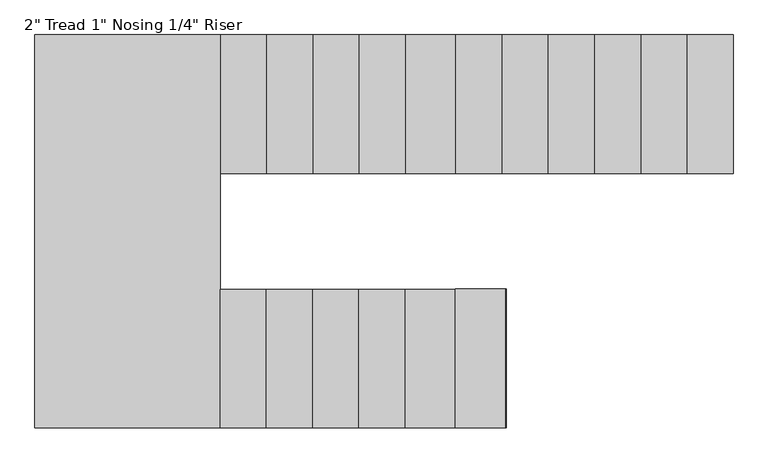
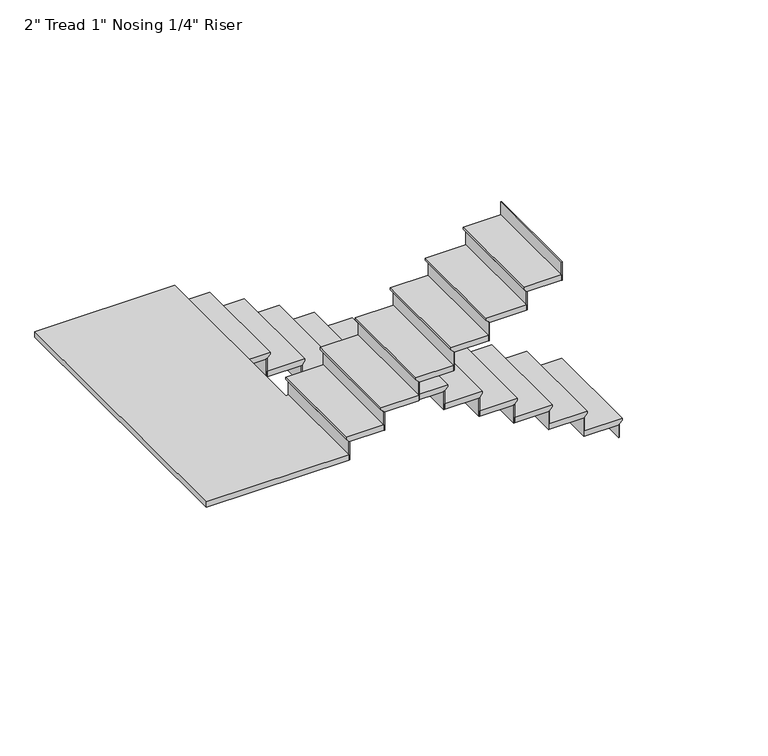
"""IFC4 building model written with IfcOpenShell, lengths in millimetres: stair flight geometry."""

from ifc_helpers import new_model, si_unit, origin, place, context, project, spatial, faceted_brep, source, transform, mapped, element, save


def stair_flight_6b31ae14(model_context):
    return source(origin(), model_context, "Body", "Brep", [
        faceted_brep([(10969.6546318, 8847.834892, 149.3921053), (10969.6546318, 8847.834892, 168.4421053), (10969.6546318, 7933.434892, 168.4421053), (10969.6546318, 7933.434892, 149.3921053), (10944.2546318, 8847.834892, 123.9921053), (10944.2546318, 7933.434892, 123.9921053), (10639.4546318, 8847.834892, 168.4421053), (10639.4546318, 7933.434892, 168.4421053), (10944.2546318, 7933.434892, 117.6421053), (10639.4546318, 7933.434892, 117.6421053), (10639.4546318, 8847.834892, 117.6421053), (10944.2546318, 8847.834892, 117.6421053)], [[[0, 1, 2, 3]], [[4, 0, 3, 5]], [[2, 1, 6, 7]], [[8, 9, 10, 11]], [[2, 7, 9, 8, 5, 3]], [[8, 11, 4, 5]], [[6, 1, 0, 4, 11, 10]], [[7, 6, 10, 9]]]),
        faceted_brep([(10944.2546318, 8847.834892, 117.6421053), (10944.2546318, 8847.834892, 0.0), (10937.9046318, 8847.834892, 0.0), (10937.9046318, 8847.834892, 117.6421053), (10944.2546318, 7933.434892, 117.6421053), (10937.9046318, 7933.434892, 117.6421053), (10937.9046318, 7933.434892, 0.0), (10944.2546318, 7933.434892, 0.0)], [[[0, 1, 2, 3]], [[4, 5, 6, 7]], [[1, 0, 4, 7]], [[2, 1, 7, 6]], [[3, 2, 6, 5]], [[0, 3, 5, 4]]]),
        faceted_brep([(10639.4546318, 8847.834892, 286.0842105), (10639.4546318, 8847.834892, 117.6421053), (10633.1046318, 8847.834892, 117.6421053), (10633.1046318, 8847.834892, 286.0842105), (10639.4546318, 7933.434892, 286.0842105), (10633.1046318, 7933.434892, 286.0842105), (10633.1046318, 7933.434892, 117.6421053), (10639.4546318, 7933.434892, 117.6421053)], [[[0, 1, 2, 3]], [[4, 5, 6, 7]], [[1, 0, 4, 7]], [[2, 1, 7, 6]], [[3, 2, 6, 5]], [[0, 3, 5, 4]]]),
        faceted_brep([(10664.8546318, 7933.434892, 336.8842105), (10664.8546318, 8847.834892, 336.8842105), (10334.6546318, 8847.834892, 336.8842105), (10334.6546318, 7933.434892, 336.8842105), (10639.4546318, 7933.434892, 286.0842105), (10334.6546318, 7933.434892, 286.0842105), (10334.6546318, 8847.834892, 286.0842105), (10639.4546318, 8847.834892, 286.0842105), (10639.4546318, 7933.434892, 292.4342105), (10664.8546318, 7933.434892, 317.8342105), (10639.4546318, 8847.834892, 292.4342105), (10664.8546318, 8847.834892, 317.8342105)], [[[0, 1, 2, 3]], [[4, 5, 6, 7]], [[0, 3, 5, 4, 8, 9]], [[4, 7, 10, 8]], [[2, 1, 11, 10, 7, 6]], [[3, 2, 6, 5]], [[11, 1, 0, 9]], [[10, 11, 9, 8]]]),
        faceted_brep([(10334.6546318, 8847.834892, 454.5263158), (10334.6546318, 8847.834892, 286.0842105), (10328.3046318, 8847.834892, 286.0842105), (10328.3046318, 8847.834892, 454.5263158), (10334.6546318, 7933.434892, 454.5263158), (10328.3046318, 7933.434892, 454.5263158), (10328.3046318, 7933.434892, 286.0842105), (10334.6546318, 7933.434892, 286.0842105)], [[[0, 1, 2, 3]], [[4, 5, 6, 7]], [[1, 0, 4, 7]], [[2, 1, 7, 6]], [[3, 2, 6, 5]], [[0, 3, 5, 4]]]),
        faceted_brep([(10360.0546318, 7933.434892, 505.3263158), (10360.0546318, 8847.834892, 505.3263158), (10029.8546318, 8847.834892, 505.3263158), (10029.8546318, 7933.434892, 505.3263158), (10334.6546318, 7933.434892, 454.5263158), (10029.8546318, 7933.434892, 454.5263158), (10029.8546318, 8847.834892, 454.5263158), (10334.6546318, 8847.834892, 454.5263158), (10334.6546318, 7933.434892, 460.8763158), (10360.0546318, 7933.434892, 486.2763158), (10334.6546318, 8847.834892, 460.8763158), (10360.0546318, 8847.834892, 486.2763158)], [[[0, 1, 2, 3]], [[4, 5, 6, 7]], [[0, 3, 5, 4, 8, 9]], [[4, 7, 10, 8]], [[2, 1, 11, 10, 7, 6]], [[3, 2, 6, 5]], [[11, 1, 0, 9]], [[10, 11, 9, 8]]]),
        faceted_brep([(10029.8546318, 8847.834892, 622.9684211), (10029.8546318, 8847.834892, 454.5263158), (10023.5046318, 8847.834892, 454.5263158), (10023.5046318, 8847.834892, 622.9684211), (10029.8546318, 7933.434892, 622.9684211), (10023.5046318, 7933.434892, 622.9684211), (10023.5046318, 7933.434892, 454.5263158), (10029.8546318, 7933.434892, 454.5263158)], [[[0, 1, 2, 3]], [[4, 5, 6, 7]], [[1, 0, 4, 7]], [[2, 1, 7, 6]], [[3, 2, 6, 5]], [[0, 3, 5, 4]]]),
        faceted_brep([(10055.2546318, 7933.434892, 673.7684211), (10055.2546318, 8847.834892, 673.7684211), (9725.0546318, 8847.834892, 673.7684211), (9725.0546318, 7933.434892, 673.7684211), (10029.8546318, 7933.434892, 622.9684211), (9725.0546318, 7933.434892, 622.9684211), (9725.0546318, 8847.834892, 622.9684211), (10029.8546318, 8847.834892, 622.9684211), (10029.8546318, 7933.434892, 629.3184211), (10055.2546318, 7933.434892, 654.7184211), (10029.8546318, 8847.834892, 629.3184211), (10055.2546318, 8847.834892, 654.7184211)], [[[0, 1, 2, 3]], [[4, 5, 6, 7]], [[0, 3, 5, 4, 8, 9]], [[4, 7, 10, 8]], [[2, 1, 11, 10, 7, 6]], [[3, 2, 6, 5]], [[11, 1, 0, 9]], [[10, 11, 9, 8]]]),
        faceted_brep([(9725.0546318, 8847.834892, 791.4105263), (9725.0546318, 8847.834892, 622.9684211), (9718.7046318, 8847.834892, 622.9684211), (9718.7046318, 8847.834892, 791.4105263), (9725.0546318, 7933.434892, 791.4105263), (9718.7046318, 7933.434892, 791.4105263), (9718.7046318, 7933.434892, 622.9684211), (9725.0546318, 7933.434892, 622.9684211)], [[[0, 1, 2, 3]], [[4, 5, 6, 7]], [[1, 0, 4, 7]], [[2, 1, 7, 6]], [[3, 2, 6, 5]], [[0, 3, 5, 4]]]),
        faceted_brep([(9750.4546318, 7933.434892, 842.2105263), (9750.4546318, 8847.834892, 842.2105263), (9420.2546318, 8847.834892, 842.2105263), (9420.2546318, 7933.434892, 842.2105263), (9725.0546318, 7933.434892, 791.4105263), (9420.2546318, 7933.434892, 791.4105263), (9420.2546318, 8847.834892, 791.4105263), (9725.0546318, 8847.834892, 791.4105263), (9725.0546318, 7933.434892, 797.7605263), (9750.4546318, 7933.434892, 823.1605263), (9725.0546318, 8847.834892, 797.7605263), (9750.4546318, 8847.834892, 823.1605263)], [[[0, 1, 2, 3]], [[4, 5, 6, 7]], [[0, 3, 5, 4, 8, 9]], [[4, 7, 10, 8]], [[2, 1, 11, 10, 7, 6]], [[3, 2, 6, 5]], [[11, 1, 0, 9]], [[10, 11, 9, 8]]]),
        faceted_brep([(9420.2546318, 8847.834892, 959.8526316), (9420.2546318, 8847.834892, 791.4105263), (9413.9046318, 8847.834892, 791.4105263), (9413.9046318, 8847.834892, 959.8526316), (9420.2546318, 7933.434892, 959.8526316), (9413.9046318, 7933.434892, 959.8526316), (9413.9046318, 7933.434892, 791.4105263), (9420.2546318, 7933.434892, 791.4105263)], [[[0, 1, 2, 3]], [[4, 5, 6, 7]], [[1, 0, 4, 7]], [[2, 1, 7, 6]], [[3, 2, 6, 5]], [[0, 3, 5, 4]]]),
        faceted_brep([(9445.6546318, 7933.434892, 1010.6526316), (9445.6546318, 8847.834892, 1010.6526316), (9115.4546318, 8847.834892, 1010.6526316), (9115.4546318, 7933.434892, 1010.6526316), (9420.2546318, 7933.434892, 959.8526316), (9115.4546318, 7933.434892, 959.8526316), (9115.4546318, 8847.834892, 959.8526316), (9420.2546318, 8847.834892, 959.8526316), (9420.2546318, 7933.434892, 966.2026316), (9445.6546318, 7933.434892, 991.6026316), (9420.2546318, 8847.834892, 966.2026316), (9445.6546318, 8847.834892, 991.6026316)], [[[0, 1, 2, 3]], [[4, 5, 6, 7]], [[0, 3, 5, 4, 8, 9]], [[4, 7, 10, 8]], [[2, 1, 11, 10, 7, 6]], [[3, 2, 6, 5]], [[11, 1, 0, 9]], [[10, 11, 9, 8]]]),
        faceted_brep([(9115.4546318, 8847.834892, 1128.2947368), (9115.4546318, 8847.834892, 959.8526316), (9109.1046318, 8847.834892, 959.8526316), (9109.1046318, 8847.834892, 1128.2947368), (9115.4546318, 7933.434892, 1128.2947368), (9109.1046318, 7933.434892, 1128.2947368), (9109.1046318, 7933.434892, 959.8526316), (9115.4546318, 7933.434892, 959.8526316)], [[[0, 1, 2, 3]], [[4, 5, 6, 7]], [[1, 0, 4, 7]], [[2, 1, 7, 6]], [[3, 2, 6, 5]], [[0, 3, 5, 4]]]),
        faceted_brep([(9140.8546318, 7933.434892, 1179.0947368), (9140.8546318, 8847.834892, 1179.0947368), (8785.2546318, 8847.834892, 1179.0947368), (8785.2546318, 7933.434892, 1179.0947368), (9115.4546318, 7933.434892, 1128.2947368), (8785.2546318, 7933.434892, 1128.2947368), (8785.2546318, 8847.834892, 1128.2947368), (9115.4546318, 8847.834892, 1128.2947368), (9115.4546318, 7933.434892, 1134.6447368), (9140.8546318, 7933.434892, 1160.0447368), (9115.4546318, 8847.834892, 1134.6447368), (9140.8546318, 8847.834892, 1160.0447368)], [[[0, 1, 2, 3]], [[4, 5, 6, 7]], [[0, 3, 5, 4, 8, 9]], [[4, 7, 10, 8]], [[2, 1, 11, 10, 7, 6]], [[3, 2, 6, 5]], [[11, 1, 0, 9]], [[10, 11, 9, 8]]]),
        faceted_brep([(8785.2546318, 8847.834892, 1296.7368421), (8785.2546318, 8847.834892, 1128.2947368), (8778.9046318, 8847.834892, 1128.2947368), (8778.9046318, 8847.834892, 1296.7368421), (8785.2546318, 7933.434892, 1296.7368421), (8778.9046318, 7933.434892, 1296.7368421), (8778.9046318, 7933.434892, 1128.2947368), (8785.2546318, 7933.434892, 1128.2947368)], [[[0, 1, 2, 3]], [[4, 5, 6, 7]], [[1, 0, 4, 7]], [[2, 1, 7, 6]], [[3, 2, 6, 5]], [[0, 3, 5, 4]]]),
        faceted_brep([(8810.6546318, 7933.434892, 1347.5368421), (8810.6546318, 8847.834892, 1347.5368421), (8480.4546318, 8847.834892, 1347.5368421), (8480.4546318, 7933.434892, 1347.5368421), (8785.2546318, 7933.434892, 1296.7368421), (8480.4546318, 7933.434892, 1296.7368421), (8480.4546318, 8847.834892, 1296.7368421), (8785.2546318, 8847.834892, 1296.7368421), (8785.2546318, 7933.434892, 1303.0868421), (8810.6546318, 7933.434892, 1328.4868421), (8785.2546318, 8847.834892, 1303.0868421), (8810.6546318, 8847.834892, 1328.4868421)], [[[0, 1, 2, 3]], [[4, 5, 6, 7]], [[0, 3, 5, 4, 8, 9]], [[4, 7, 10, 8]], [[2, 1, 11, 10, 7, 6]], [[3, 2, 6, 5]], [[11, 1, 0, 9]], [[10, 11, 9, 8]]]),
        faceted_brep([(8480.4546318, 8847.834892, 1465.1789474), (8480.4546318, 8847.834892, 1296.7368421), (8474.1046318, 8847.834892, 1296.7368421), (8474.1046318, 8847.834892, 1465.1789474), (8480.4546318, 7933.434892, 1465.1789474), (8474.1046318, 7933.434892, 1465.1789474), (8474.1046318, 7933.434892, 1296.7368421), (8480.4546318, 7933.434892, 1296.7368421)], [[[0, 1, 2, 3]], [[4, 5, 6, 7]], [[1, 0, 4, 7]], [[2, 1, 7, 6]], [[3, 2, 6, 5]], [[0, 3, 5, 4]]]),
        faceted_brep([(8505.8546318, 7933.434892, 1515.9789474), (8505.8546318, 8847.834892, 1515.9789474), (8175.6546318, 8847.834892, 1515.9789474), (8175.6546318, 7933.434892, 1515.9789474), (8480.4546318, 7933.434892, 1465.1789474), (8175.6546318, 7933.434892, 1465.1789474), (8175.6546318, 8847.834892, 1465.1789474), (8480.4546318, 8847.834892, 1465.1789474), (8480.4546318, 7933.434892, 1471.5289474), (8505.8546318, 7933.434892, 1496.9289474), (8480.4546318, 8847.834892, 1471.5289474), (8505.8546318, 8847.834892, 1496.9289474)], [[[0, 1, 2, 3]], [[4, 5, 6, 7]], [[0, 3, 5, 4, 8, 9]], [[4, 7, 10, 8]], [[2, 1, 11, 10, 7, 6]], [[3, 2, 6, 5]], [[11, 1, 0, 9]], [[10, 11, 9, 8]]]),
        faceted_brep([(8175.6546318, 8847.834892, 1633.6210526), (8175.6546318, 8847.834892, 1465.1789474), (8169.3046318, 8847.834892, 1465.1789474), (8169.3046318, 8847.834892, 1633.6210526), (8175.6546318, 7933.434892, 1633.6210526), (8169.3046318, 7933.434892, 1633.6210526), (8169.3046318, 7933.434892, 1465.1789474), (8175.6546318, 7933.434892, 1465.1789474)], [[[0, 1, 2, 3]], [[4, 5, 6, 7]], [[1, 0, 4, 7]], [[2, 1, 7, 6]], [[3, 2, 6, 5]], [[0, 3, 5, 4]]]),
        faceted_brep([(8201.0546318, 7933.434892, 1684.4210526), (8201.0546318, 8847.834892, 1684.4210526), (7870.8546318, 8847.834892, 1684.4210526), (7870.8546318, 7933.434892, 1684.4210526), (8175.6546318, 7933.434892, 1633.6210526), (7870.8546318, 7933.434892, 1633.6210526), (7870.8546318, 8847.834892, 1633.6210526), (8175.6546318, 8847.834892, 1633.6210526), (8175.6546318, 7933.434892, 1639.9710526), (8201.0546318, 7933.434892, 1665.3710526), (8175.6546318, 8847.834892, 1639.9710526), (8201.0546318, 8847.834892, 1665.3710526)], [[[0, 1, 2, 3]], [[4, 5, 6, 7]], [[0, 3, 5, 4, 8, 9]], [[4, 7, 10, 8]], [[2, 1, 11, 10, 7, 6]], [[3, 2, 6, 5]], [[11, 1, 0, 9]], [[10, 11, 9, 8]]]),
        faceted_brep([(7870.8546318, 8847.834892, 1802.0631579), (7870.8546318, 8847.834892, 1633.6210526), (7864.5046318, 8847.834892, 1633.6210526), (7864.5046318, 8847.834892, 1802.0631579), (7870.8546318, 7933.434892, 1802.0631579), (7864.5046318, 7933.434892, 1802.0631579), (7864.5046318, 7933.434892, 1633.6210526), (7870.8546318, 7933.434892, 1633.6210526)], [[[0, 1, 2, 3]], [[4, 5, 6, 7]], [[1, 0, 4, 7]], [[2, 1, 7, 6]], [[3, 2, 6, 5]], [[0, 3, 5, 4]]]),
        faceted_brep([(7896.2546318, 7933.434892, 1852.8631579), (7896.2546318, 8847.834892, 1852.8631579), (7566.0546318, 8847.834892, 1852.8631579), (7566.0546318, 7933.434892, 1852.8631579), (7870.8546318, 7933.434892, 1802.0631579), (7566.0546318, 7933.434892, 1802.0631579), (7566.0546318, 8847.834892, 1802.0631579), (7870.8546318, 8847.834892, 1802.0631579), (7870.8546318, 7933.434892, 1808.4131579), (7896.2546318, 7933.434892, 1833.8131579), (7870.8546318, 8847.834892, 1808.4131579), (7896.2546318, 8847.834892, 1833.8131579)], [[[0, 1, 2, 3]], [[4, 5, 6, 7]], [[0, 3, 5, 4, 8, 9]], [[4, 7, 10, 8]], [[2, 1, 11, 10, 7, 6]], [[3, 2, 6, 5]], [[11, 1, 0, 9]], [[10, 11, 9, 8]]]),
        faceted_brep([(7566.0546318, 8847.834892, 1970.5052632), (7566.0546318, 8847.834892, 1802.0631579), (7559.7046318, 8847.834892, 1802.0631579), (7559.7046318, 8847.834892, 1970.5052632), (7566.0546318, 7933.434892, 1970.5052632), (7559.7046318, 7933.434892, 1970.5052632), (7559.7046318, 7933.434892, 1802.0631579), (7566.0546318, 7933.434892, 1802.0631579)], [[[0, 1, 2, 3]], [[4, 5, 6, 7]], [[1, 0, 4, 7]], [[2, 1, 7, 6]], [[3, 2, 6, 5]], [[0, 3, 5, 4]]]),
        faceted_brep([(7616.8546318, 7171.434892, 2021.3052632), (7591.4546318, 7171.434892, 2021.3052632), (7591.4546318, 8847.834892, 2021.3052632), (6372.2546318, 8847.834892, 2021.3052632), (6372.2546318, 6257.034892, 2021.3052632), (7616.8546318, 6257.034892, 2021.3052632), (7591.4546318, 7171.434892, 1970.5052632), (7616.8546318, 7171.434892, 1970.5052632), (7616.8546318, 6257.034892, 1970.5052632), (6372.2546318, 6257.034892, 1970.5052632), (6372.2546318, 8847.834892, 1970.5052632), (7566.0546318, 8847.834892, 1970.5052632), (7566.0546318, 7933.434892, 1970.5052632), (7591.4546318, 7933.434892, 1970.5052632), (7591.4546318, 7933.434892, 2002.2552632), (7591.4546318, 8847.834892, 2002.2552632), (7566.0546318, 7933.434892, 1976.8552632), (7566.0546318, 8847.834892, 1976.8552632)], [[[0, 1, 2, 3, 4, 5]], [[6, 7, 8, 9, 10, 11, 12, 13]], [[1, 0, 7, 6]], [[2, 1, 6, 13, 14, 15]], [[13, 12, 16, 14]], [[12, 11, 17, 16]], [[3, 2, 15, 17, 11, 10]], [[4, 3, 10, 9]], [[5, 4, 9, 8]], [[0, 5, 8, 7]], [[17, 15, 14, 16]]]),
        faceted_brep([(7616.8546318, 6257.034892, 2138.9473684), (7616.8546318, 6257.034892, 1970.5052632), (7623.2046318, 6257.034892, 1970.5052632), (7623.2046318, 6257.034892, 2138.9473684), (7616.8546318, 7171.434892, 2138.9473684), (7623.2046318, 7171.434892, 2138.9473684), (7623.2046318, 7171.434892, 1970.5052632), (7616.8546318, 7171.434892, 1970.5052632)], [[[0, 1, 2, 3]], [[4, 5, 6, 7]], [[1, 0, 4, 7]], [[2, 1, 7, 6]], [[3, 2, 6, 5]], [[0, 3, 5, 4]]]),
        faceted_brep([(7591.4546318, 7171.434892, 2189.7473684), (7591.4546318, 6257.034892, 2189.7473684), (7921.6546318, 6257.034892, 2189.7473684), (7921.6546318, 7171.434892, 2189.7473684), (7616.8546318, 7171.434892, 2138.9473684), (7921.6546318, 7171.434892, 2138.9473684), (7921.6546318, 6257.034892, 2138.9473684), (7616.8546318, 6257.034892, 2138.9473684), (7616.8546318, 7171.434892, 2145.2973684), (7591.4546318, 7171.434892, 2170.6973684), (7616.8546318, 6257.034892, 2145.2973684), (7591.4546318, 6257.034892, 2170.6973684)], [[[0, 1, 2, 3]], [[4, 5, 6, 7]], [[0, 3, 5, 4, 8, 9]], [[4, 7, 10, 8]], [[2, 1, 11, 10, 7, 6]], [[3, 2, 6, 5]], [[11, 1, 0, 9]], [[10, 11, 9, 8]]]),
        faceted_brep([(7921.6546318, 6257.034892, 2307.3894737), (7921.6546318, 6257.034892, 2138.9473684), (7928.0046318, 6257.034892, 2138.9473684), (7928.0046318, 6257.034892, 2307.3894737), (7921.6546318, 7171.434892, 2307.3894737), (7928.0046318, 7171.434892, 2307.3894737), (7928.0046318, 7171.434892, 2138.9473684), (7921.6546318, 7171.434892, 2138.9473684)], [[[0, 1, 2, 3]], [[4, 5, 6, 7]], [[1, 0, 4, 7]], [[2, 1, 7, 6]], [[3, 2, 6, 5]], [[0, 3, 5, 4]]]),
        faceted_brep([(7896.2546318, 7171.434892, 2358.1894737), (7896.2546318, 6257.034892, 2358.1894737), (8226.4546318, 6257.034892, 2358.1894737), (8226.4546318, 7171.434892, 2358.1894737), (7921.6546318, 7171.434892, 2307.3894737), (8226.4546318, 7171.434892, 2307.3894737), (8226.4546318, 6257.034892, 2307.3894737), (7921.6546318, 6257.034892, 2307.3894737), (7921.6546318, 7171.434892, 2313.7394737), (7896.2546318, 7171.434892, 2339.1394737), (7921.6546318, 6257.034892, 2313.7394737), (7896.2546318, 6257.034892, 2339.1394737)], [[[0, 1, 2, 3]], [[4, 5, 6, 7]], [[0, 3, 5, 4, 8, 9]], [[4, 7, 10, 8]], [[2, 1, 11, 10, 7, 6]], [[3, 2, 6, 5]], [[11, 1, 0, 9]], [[10, 11, 9, 8]]]),
        faceted_brep([(8226.4546318, 6257.034892, 2475.8315789), (8226.4546318, 6257.034892, 2307.3894737), (8232.8046318, 6257.034892, 2307.3894737), (8232.8046318, 6257.034892, 2475.8315789), (8226.4546318, 7171.434892, 2475.8315789), (8232.8046318, 7171.434892, 2475.8315789), (8232.8046318, 7171.434892, 2307.3894737), (8226.4546318, 7171.434892, 2307.3894737)], [[[0, 1, 2, 3]], [[4, 5, 6, 7]], [[1, 0, 4, 7]], [[2, 1, 7, 6]], [[3, 2, 6, 5]], [[0, 3, 5, 4]]]),
        faceted_brep([(8201.0546318, 7171.434892, 2526.6315789), (8201.0546318, 6257.034892, 2526.6315789), (8531.2546318, 6257.034892, 2526.6315789), (8531.2546318, 7171.434892, 2526.6315789), (8226.4546318, 7171.434892, 2475.8315789), (8531.2546318, 7171.434892, 2475.8315789), (8531.2546318, 6257.034892, 2475.8315789), (8226.4546318, 6257.034892, 2475.8315789), (8226.4546318, 7171.434892, 2482.1815789), (8201.0546318, 7171.434892, 2507.5815789), (8226.4546318, 6257.034892, 2482.1815789), (8201.0546318, 6257.034892, 2507.5815789)], [[[0, 1, 2, 3]], [[4, 5, 6, 7]], [[0, 3, 5, 4, 8, 9]], [[4, 7, 10, 8]], [[2, 1, 11, 10, 7, 6]], [[3, 2, 6, 5]], [[11, 1, 0, 9]], [[10, 11, 9, 8]]]),
        faceted_brep([(8531.2546318, 6257.034892, 2644.2736842), (8531.2546318, 6257.034892, 2475.8315789), (8537.6046318, 6257.034892, 2475.8315789), (8537.6046318, 6257.034892, 2644.2736842), (8531.2546318, 7171.434892, 2644.2736842), (8537.6046318, 7171.434892, 2644.2736842), (8537.6046318, 7171.434892, 2475.8315789), (8531.2546318, 7171.434892, 2475.8315789)], [[[0, 1, 2, 3]], [[4, 5, 6, 7]], [[1, 0, 4, 7]], [[2, 1, 7, 6]], [[3, 2, 6, 5]], [[0, 3, 5, 4]]]),
        faceted_brep([(8505.8546318, 7171.434892, 2695.0736842), (8505.8546318, 6257.034892, 2695.0736842), (8836.0546318, 6257.034892, 2695.0736842), (8836.0546318, 7171.434892, 2695.0736842), (8531.2546318, 7171.434892, 2644.2736842), (8836.0546318, 7171.434892, 2644.2736842), (8836.0546318, 6257.034892, 2644.2736842), (8531.2546318, 6257.034892, 2644.2736842), (8531.2546318, 7171.434892, 2650.6236842), (8505.8546318, 7171.434892, 2676.0236842), (8531.2546318, 6257.034892, 2650.6236842), (8505.8546318, 6257.034892, 2676.0236842)], [[[0, 1, 2, 3]], [[4, 5, 6, 7]], [[0, 3, 5, 4, 8, 9]], [[4, 7, 10, 8]], [[2, 1, 11, 10, 7, 6]], [[3, 2, 6, 5]], [[11, 1, 0, 9]], [[10, 11, 9, 8]]]),
        faceted_brep([(8836.0546318, 6257.034892, 2812.7157895), (8836.0546318, 6257.034892, 2644.2736842), (8842.4046318, 6257.034892, 2644.2736842), (8842.4046318, 6257.034892, 2812.7157895), (8836.0546318, 7171.434892, 2812.7157895), (8842.4046318, 7171.434892, 2812.7157895), (8842.4046318, 7171.434892, 2644.2736842), (8836.0546318, 7171.434892, 2644.2736842)], [[[0, 1, 2, 3]], [[4, 5, 6, 7]], [[1, 0, 4, 7]], [[2, 1, 7, 6]], [[3, 2, 6, 5]], [[0, 3, 5, 4]]]),
        faceted_brep([(8810.6546318, 7171.434892, 2863.5157895), (8810.6546318, 6257.034892, 2863.5157895), (9166.2546318, 6257.034892, 2863.5157895), (9166.2546318, 7171.434892, 2863.5157895), (8836.0546318, 7171.434892, 2812.7157895), (9166.2546318, 7171.434892, 2812.7157895), (9166.2546318, 6257.034892, 2812.7157895), (8836.0546318, 6257.034892, 2812.7157895), (8836.0546318, 7171.434892, 2819.0657895), (8810.6546318, 7171.434892, 2844.4657895), (8836.0546318, 6257.034892, 2819.0657895), (8810.6546318, 6257.034892, 2844.4657895)], [[[0, 1, 2, 3]], [[4, 5, 6, 7]], [[0, 3, 5, 4, 8, 9]], [[4, 7, 10, 8]], [[2, 1, 11, 10, 7, 6]], [[3, 2, 6, 5]], [[11, 1, 0, 9]], [[10, 11, 9, 8]]]),
        faceted_brep([(9166.2546318, 6257.034892, 2981.1578947), (9166.2546318, 6257.034892, 2812.7157895), (9172.6046318, 6257.034892, 2812.7157895), (9172.6046318, 6257.034892, 2981.1578947), (9166.2546318, 7171.434892, 2981.1578947), (9172.6046318, 7171.434892, 2981.1578947), (9172.6046318, 7171.434892, 2812.7157895), (9166.2546318, 7171.434892, 2812.7157895)], [[[0, 1, 2, 3]], [[4, 5, 6, 7]], [[1, 0, 4, 7]], [[2, 1, 7, 6]], [[3, 2, 6, 5]], [[0, 3, 5, 4]]]),
        faceted_brep([(9140.8546318, 7171.434892, 3031.9578947), (9140.8546318, 6257.034892, 3031.9578947), (9471.0546318, 6257.034892, 3031.9578947), (9471.0546318, 7171.434892, 3031.9578947), (9166.2546318, 7171.434892, 2981.1578947), (9471.0546318, 7171.434892, 2981.1578947), (9471.0546318, 6257.034892, 2981.1578947), (9166.2546318, 6257.034892, 2981.1578947), (9166.2546318, 7171.434892, 2987.5078947), (9140.8546318, 7171.434892, 3012.9078947), (9166.2546318, 6257.034892, 2987.5078947), (9140.8546318, 6257.034892, 3012.9078947)], [[[0, 1, 2, 3]], [[4, 5, 6, 7]], [[0, 3, 5, 4, 8, 9]], [[4, 7, 10, 8]], [[2, 1, 11, 10, 7, 6]], [[3, 2, 6, 5]], [[11, 1, 0, 9]], [[10, 11, 9, 8]]]),
        faceted_brep([(9471.0546318, 6257.034892, 3149.6), (9471.0546318, 6257.034892, 2981.1578947), (9477.4046318, 6257.034892, 2981.1578947), (9477.4046318, 6257.034892, 3149.6), (9471.0546318, 7171.434892, 3149.6), (9477.4046318, 7171.434892, 3149.6), (9477.4046318, 7171.434892, 2981.1578947), (9471.0546318, 7171.434892, 2981.1578947)], [[[0, 1, 2, 3]], [[4, 5, 6, 7]], [[1, 0, 4, 7]], [[2, 1, 7, 6]], [[3, 2, 6, 5]], [[0, 3, 5, 4]]]),
    ])


if __name__ == "__main__":
    model = new_model("IFC4")
    model_context = context("Model", 3, world=origin())
    ifc_project = project(units=[si_unit("LENGTHUNIT", "METRE", prefix="MILLI")], contexts=[model_context])
    site = spatial("IfcSite", under=ifc_project)
    building = spatial("IfcBuilding", under=site)
    placement = place(None, origin())
    stair_flight_shape = stair_flight_6b31ae14(model_context)
    element("IfcStairFlight", 1, ObjectType="2\" Tread 1\" Nosing 1/4\" Riser", at=placement, inside=building, context=model_context, shape_type="MappedRepresentation", body=[
        mapped(stair_flight_shape, transform((0.0, 0.0, 0.0), x_axis=(1.0, 0.0, 0.0), y_axis=(0.0, 1.0, 0.0), z_axis=(0.0, 0.0, 1.0))),
    ])
    save(model, "model.ifc")
